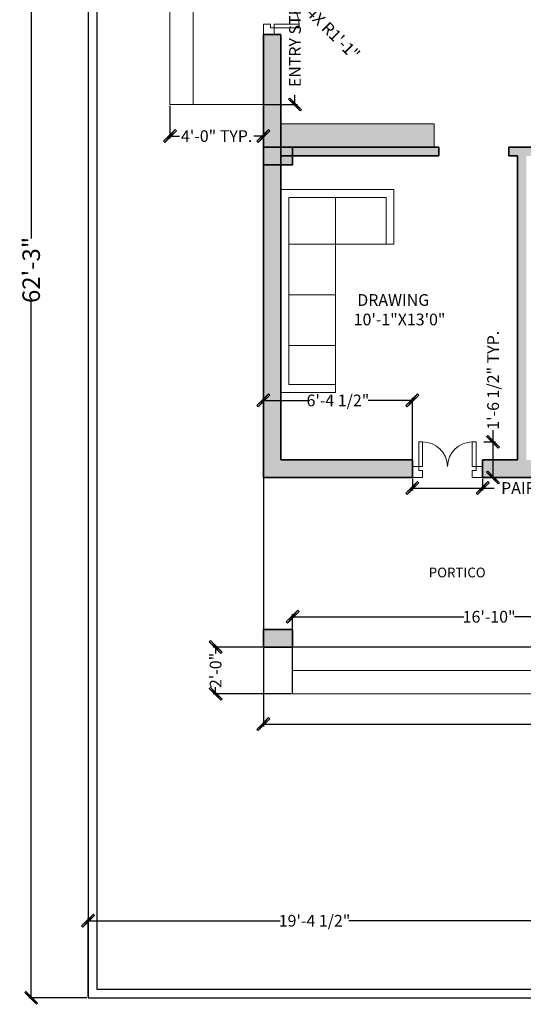
# Model space of a CAD drawing. Units: inches. Extents: x 1018 to 2596, y 723 to 1501.
# Tile 1 of 6: x 1018 to 1276, y 723 to 1229. Entities that reach past the tile are written whole.
import ezdxf

# ---------------------------------------------------------------- set-up
doc = ezdxf.new("R2010")
doc.units = ezdxf.units.IN
doc.layers.get('Defpoints').update_dxf_attribs({"lineweight": 0})
for name, color, linetype, lineweight in [('A-ANNO-DIMS', 2, 'Continuous', 13), ('A-AREA-IDEN', 7, 'Continuous', 18), ('A-COLS', 7, 'Continuous', 35), ('A-DOOR', 4, 'Continuous', 18), ('A-FLOR', 7, 'Continuous', 25), ('A-FLOR-CASE', 8, 'Continuous', 18), ('A-FLOR-CASE-PATT', 9, 'Continuous', 9), ('A-FLOR-STRS', 7, 'Continuous', 18), ('A-FURN', 8, 'Continuous', 13), ('A-WALL', 7, 'Continuous', 35), ('C-PROP', 7, 'Continuous', 25)]:
    doc.layers.add(name, color=color, linetype=linetype, lineweight=lineweight)
doc.layers.add('A-WALL-PATT', color=9, linetype='Continuous', lineweight=9, true_color=0xc7c8ca)
doc.styles.get("Standard").update_dxf_attribs({"font": 'arial.ttf'})
doc.dimstyles.new('saketh', dxfattribs={"dimtxt": 6, "dimasz": 6, "dimexe": 1.25, "dimexo": 0.625, "dimtad": 0, "dimdec": 1, "dimlunit": 4, "dimtxsty": 'Standard', "dimblk": 'ARCHTICK', "dimcen": 2.5, "dimclrd": 256, "dimclre": 1, "dimadec": 0, "dimazin": 0, "dimtfac": 1, "dimtdec": 1, "dimtmove": 0, "dimatfit": 3, "dimldrblk": 'ARCHTICK', "dimfxl": 1, "dimtolj": 1, "dimarcsym": 0})

# ---------------------------------------------------------------- blocks, each defined once
blk = doc.blocks.new('3 1')
at = {"layer": 'A-DOOR'}
for points in [[(-32.72, 5.56), (-32.72, 18.28), (-30.75, 18.28), (-30.75, 5.56)], [(-3.28, 5.56), (-3.28, 18.28), (-5.25, 18.28), (-5.25, 5.56)], [(-32.72, 5.56), (-36, 5.56), (-36, 0), (-30.75, 0), (-30.75, 3.59), (-32.72, 3.59)], [(-5.25, 3.59), (-5.25, 0), (0, 0), (0, 5.56), (-3.28, 5.56), (-3.28, 3.59)]]:
    blk.add_lwpolyline(points, close=True, dxfattribs=at)
at = {"layer": 'A-DOOR', "ltscale": 0.1}
for centre, start, end in [((-30.75, 5.53), 0.1406, 90), ((-5.25, 5.53), 90, 179.8594)]:
    blk.add_arc(centre, 12.75, start, end, dxfattribs=at)
blk = doc.blocks.new('_ArchTick')
for p, q in [((0.447, 0.553), (-0.553, -0.447)), ((-0.447, -0.553), (0.553, 0.447)), ((0.553, 0.447), (0.447, 0.553)), ((-0.553, -0.447), (-0.447, -0.553))]:
    blk.add_line(p, q)
mesh = blk.add_polyface()
corners = [(-0.447, -0.553), (0.447, 0.553), (-0.553, -0.447), (0.553, 0.447)]
mesh.append_faces([[corners[k] for k in face] for face in [(0, 1, 2), (1, 0, 3)]], dxfattribs={"vtx0": -1})
blk = doc.blocks.new('*D49')
at = {"layer": 'A-ANNO-DIMS', "color": 0, "lineweight": -2, "transparency": 16777216}
for p, q in [((1052.06, 1473.73), (1022.21, 1473.73)), ((1023.46, 1473.73), (1023.46, 1116.33)), ((1023.46, 726.73), (1023.46, 1084.12)), ((1052.06, 726.73), (1022.21, 726.73))]:
    blk.add_line(p, q, dxfattribs=at)
at = {"layer": 'Defpoints', "color": 0, "transparency": 16777216}
for p in [(1052.69, 1473.73), (1023.46, 726.73), (1052.69, 726.73)]:
    blk.add_point(p, dxfattribs=at)
at = {"layer": 'A-ANNO-DIMS', "color": 0, "lineweight": -2, "transparency": 16777216, "xscale": 6, "yscale": 6, "zscale": 6}
for p, rotation in [((1023.46, 1473.73), 90), ((1023.46, 726.73), 270)]:
    blk.add_blockref('_ArchTick', p, dxfattribs=dict(at, rotation=rotation))
at = {"layer": 'A-ANNO-DIMS', "color": 0, "transparency": 16777216, "insert": (1023.46, 1100.23), "char_height": 9, "attachment_point": 5, "rotation": 90}
blk.add_mtext('\\A1;62\'-3"', dxfattribs=at)
blk = doc.blocks.new('COLUMN-15X9-IN')
h = blk.add_hatch(color=256)
h.dxf.hatch_style = 1
h.paths.add_polyline_path([(15, 0), (15, 9), (0, 9), (0, 0)])
blk.add_lwpolyline([(15, 9), (15, 0), (0, 0), (0, 9)], close=True)
blk = doc.blocks.new('ENTRY-STEP-108X48-IN')
for p, q in [((0, 0), (0, 108)), ((0, 108), (12, 108)), ((12, 0), (12, 108)), ((48, 108), (12, 108)), ((0, 0), (12, 0)), ((48, 0), (12, 0))]:
    blk.add_line(p, q)
blk = doc.blocks.new('*D59')
at = {"layer": 'A-ANNO-DIMS', "color": 1, "lineweight": -2, "transparency": 16777216}
for p, q in [((1219.19, 993.1), (1219.19, 987.08)), ((1255.19, 993.1), (1255.19, 987.08))]:
    blk.add_line(p, q, dxfattribs=at)
at = {"layer": 'A-ANNO-DIMS', "lineweight": -2, "transparency": 16777216}
for p, q in [((1219.19, 988.33), (1255.19, 988.33)), ((1255.19, 988.33), (1261.19, 988.33))]:
    blk.add_line(p, q, dxfattribs=at)
at = {"layer": 'Defpoints', "color": 0, "transparency": 16777216}
for p in [(1219.19, 993.73), (1255.19, 993.73), (1255.19, 988.33)]:
    blk.add_point(p, dxfattribs=at)
at = {"layer": 'A-ANNO-DIMS', "lineweight": -2, "transparency": 16777216, "xscale": 6, "yscale": 6, "zscale": 6, "rotation": 180}
blk.add_blockref('_ArchTick', (1219.19, 988.33), dxfattribs=at)
at = {"layer": 'A-ANNO-DIMS', "lineweight": -2, "transparency": 16777216, "xscale": 6, "yscale": 6, "zscale": 6}
blk.add_blockref('_ArchTick', (1255.19, 988.33), dxfattribs=at)
at = {"layer": 'A-ANNO-DIMS', "color": 0, "transparency": 16777216, "insert": (1310.45, 988.33), "char_height": 6, "attachment_point": 5}
blk.add_mtext('\\A1;PAIRED DOOR 3\'-0" TYP.', dxfattribs=at)
blk = doc.blocks.new('*D60')
at = {"layer": 'A-ANNO-DIMS', "lineweight": -2, "transparency": 16777216}
for p, q in [((1260.59, 1012.01), (1260.59, 1018.01)), ((1260.59, 993.73), (1260.59, 1012.01))]:
    blk.add_line(p, q, dxfattribs=at)
at = {"layer": 'A-ANNO-DIMS', "color": 1, "lineweight": -2, "transparency": 16777216}
for p, q in [((1255.81, 1012.01), (1261.84, 1012.01)), ((1255.81, 993.73), (1261.84, 993.73))]:
    blk.add_line(p, q, dxfattribs=at)
at = {"layer": 'Defpoints', "color": 0, "transparency": 16777216}
for p in [(1255.19, 1012.01), (1260.59, 1012.01), (1255.19, 993.73)]:
    blk.add_point(p, dxfattribs=at)
at = {"layer": 'A-ANNO-DIMS', "lineweight": -2, "transparency": 16777216, "xscale": 6, "yscale": 6, "zscale": 6}
for p, rotation in [((1260.59, 1012.01), 90), ((1260.59, 993.73), 270)]:
    blk.add_blockref('_ArchTick', p, dxfattribs=dict(at, rotation=rotation))
at = {"layer": 'A-ANNO-DIMS', "color": 0, "transparency": 16777216, "insert": (1260.59, 1043.63), "char_height": 6, "attachment_point": 5, "rotation": 90}
blk.add_mtext('\\A1;1\'-6 1/2" TYP.', dxfattribs=at)
blk = doc.blocks.new('*D69')
at = {"layer": 'A-ANNO-DIMS', "color": 1, "lineweight": -2, "transparency": 16777216}
for p, q in [((1143.31, 1293.11), (1160.14, 1293.11)), ((1143.31, 1185.11), (1160.14, 1185.11))]:
    blk.add_line(p, q, dxfattribs=at)
at = {"layer": 'A-ANNO-DIMS', "lineweight": -2, "transparency": 16777216}
for p, q in [((1158.89, 1293.11), (1158.89, 1288.14)), ((1158.89, 1185.11), (1158.89, 1190.09))]:
    blk.add_line(p, q, dxfattribs=at)
at = {"layer": 'Defpoints', "color": 0, "transparency": 16777216}
for p in [(1142.69, 1293.11), (1158.89, 1293.11), (1142.69, 1185.11)]:
    blk.add_point(p, dxfattribs=at)
at = {"layer": 'A-ANNO-DIMS', "lineweight": -2, "transparency": 16777216, "xscale": 6, "yscale": 6, "zscale": 6}
for p, rotation in [((1158.89, 1293.11), 90), ((1158.89, 1185.11), 270)]:
    blk.add_blockref('_ArchTick', p, dxfattribs=dict(at, rotation=rotation))
at = {"layer": 'A-ANNO-DIMS', "color": 0, "transparency": 16777216, "insert": (1158.89, 1239.11), "char_height": 6, "attachment_point": 5, "rotation": 90}
blk.add_mtext('\\A1;ENTRY STEPS 9\'-0" TYP.', dxfattribs=at)
blk = doc.blocks.new('*D70')
at = {"layer": 'A-ANNO-DIMS', "color": 1, "lineweight": -2, "transparency": 16777216}
for p, q in [((1094.69, 1184.49), (1094.69, 1167.66)), ((1142.69, 1184.49), (1142.69, 1167.66))]:
    blk.add_line(p, q, dxfattribs=at)
at = {"layer": 'A-ANNO-DIMS', "lineweight": -2, "transparency": 16777216}
for p, q in [((1094.69, 1168.91), (1099.65, 1168.91)), ((1142.69, 1168.91), (1137.72, 1168.91))]:
    blk.add_line(p, q, dxfattribs=at)
at = {"layer": 'Defpoints', "color": 0, "transparency": 16777216}
for p in [(1094.69, 1185.11), (1142.69, 1185.11), (1142.69, 1168.91)]:
    blk.add_point(p, dxfattribs=at)
at = {"layer": 'A-ANNO-DIMS', "lineweight": -2, "transparency": 16777216, "xscale": 6, "yscale": 6, "zscale": 6, "rotation": 180}
blk.add_blockref('_ArchTick', (1094.69, 1168.91), dxfattribs=at)
at = {"layer": 'A-ANNO-DIMS', "lineweight": -2, "transparency": 16777216, "xscale": 6, "yscale": 6, "zscale": 6}
blk.add_blockref('_ArchTick', (1142.69, 1168.91), dxfattribs=at)
at = {"layer": 'A-ANNO-DIMS', "color": 0, "transparency": 16777216, "insert": (1118.69, 1168.91), "char_height": 6, "attachment_point": 5}
blk.add_mtext('\\A1;4\'-0" TYP.', dxfattribs=at)
blk = doc.blocks.new('*D79')
at = {"layer": 'A-ANNO-DIMS', "color": 1, "lineweight": -2, "transparency": 16777216}
for p, q in [((1142.69, 906.1), (1142.69, 865.93)), ((1583.69, 906.1), (1583.69, 865.93))]:
    blk.add_line(p, q, dxfattribs=at)
at = {"layer": 'A-ANNO-DIMS', "lineweight": -2, "transparency": 16777216}
for p, q in [((1142.69, 867.18), (1352.26, 867.18)), ((1583.69, 867.18), (1374.12, 867.18))]:
    blk.add_line(p, q, dxfattribs=at)
at = {"layer": 'Defpoints', "color": 0, "transparency": 16777216}
for p in [(1142.69, 906.73), (1583.69, 906.73), (1142.69, 867.18)]:
    blk.add_point(p, dxfattribs=at)
at = {"layer": 'A-ANNO-DIMS', "lineweight": -2, "transparency": 16777216, "xscale": 6, "yscale": 6, "zscale": 6, "rotation": 180}
blk.add_blockref('_ArchTick', (1142.69, 867.18), dxfattribs=at)
at = {"layer": 'A-ANNO-DIMS', "lineweight": -2, "transparency": 16777216, "xscale": 6, "yscale": 6, "zscale": 6}
blk.add_blockref('_ArchTick', (1583.69, 867.18), dxfattribs=at)
at = {"layer": 'A-ANNO-DIMS', "color": 0, "transparency": 16777216, "insert": (1363.19, 867.18), "char_height": 6, "attachment_point": 5}
blk.add_mtext('\\A1;36\'-9"', dxfattribs=at)
blk = doc.blocks.new('*D82')
at = {"layer": 'A-ANNO-DIMS', "color": 1, "lineweight": -2, "transparency": 16777216}
for p, q in [((1052.69, 727.35), (1052.69, 767.53)), ((1285.19, 727.35), (1285.19, 767.53))]:
    blk.add_line(p, q, dxfattribs=at)
at = {"layer": 'A-ANNO-DIMS', "lineweight": -2, "transparency": 16777216}
for p, q in [((1052.69, 766.28), (1151.3, 766.28)), ((1285.19, 766.28), (1186.58, 766.28))]:
    blk.add_line(p, q, dxfattribs=at)
at = {"layer": 'Defpoints', "color": 0, "transparency": 16777216}
for p in [(1285.19, 766.28), (1052.69, 726.73), (1285.19, 726.73)]:
    blk.add_point(p, dxfattribs=at)
at = {"layer": 'A-ANNO-DIMS', "lineweight": -2, "transparency": 16777216, "xscale": 6, "yscale": 6, "zscale": 6, "rotation": 180}
blk.add_blockref('_ArchTick', (1052.69, 766.28), dxfattribs=at)
at = {"layer": 'A-ANNO-DIMS', "lineweight": -2, "transparency": 16777216, "xscale": 6, "yscale": 6, "zscale": 6}
blk.add_blockref('_ArchTick', (1285.19, 766.28), dxfattribs=at)
at = {"layer": 'A-ANNO-DIMS', "color": 0, "transparency": 16777216, "insert": (1168.94, 766.28), "char_height": 6, "attachment_point": 5}
blk.add_mtext('\\A1;19\'-4 1/2"', dxfattribs=at)
blk = doc.blocks.new('*D84')
at = {"layer": 'A-ANNO-DIMS', "color": 1, "lineweight": -2, "transparency": 16777216}
for p, q in [((1157.69, 883.35), (1157.69, 923.53)), ((1359.46, 883.35), (1359.46, 923.53))]:
    blk.add_line(p, q, dxfattribs=at)
at = {"layer": 'A-ANNO-DIMS', "lineweight": -2, "transparency": 16777216}
for p, q in [((1157.69, 922.28), (1245.6, 922.28)), ((1359.46, 922.28), (1271.55, 922.28))]:
    blk.add_line(p, q, dxfattribs=at)
at = {"layer": 'Defpoints', "color": 0, "transparency": 16777216}
for p in [(1359.46, 922.28), (1157.69, 882.73), (1359.46, 882.73)]:
    blk.add_point(p, dxfattribs=at)
at = {"layer": 'A-ANNO-DIMS', "lineweight": -2, "transparency": 16777216, "xscale": 6, "yscale": 6, "zscale": 6, "rotation": 180}
blk.add_blockref('_ArchTick', (1157.69, 922.28), dxfattribs=at)
at = {"layer": 'A-ANNO-DIMS', "lineweight": -2, "transparency": 16777216, "xscale": 6, "yscale": 6, "zscale": 6}
blk.add_blockref('_ArchTick', (1359.46, 922.28), dxfattribs=at)
at = {"layer": 'A-ANNO-DIMS', "color": 0, "transparency": 16777216, "insert": (1258.57, 922.28), "char_height": 6, "attachment_point": 5}
blk.add_mtext('\\A1;16\'-10"', dxfattribs=at)
blk = doc.blocks.new('*D85')
at = {"layer": 'A-ANNO-DIMS', "color": 1, "lineweight": -2, "transparency": 16777216}
for p, q in [((1157.06, 906.73), (1116.89, 906.73)), ((1157.06, 882.73), (1116.89, 882.73))]:
    blk.add_line(p, q, dxfattribs=at)
at = {"layer": 'A-ANNO-DIMS', "lineweight": -2, "transparency": 16777216}
for p, q in [((1118.14, 906.73), (1118.14, 903.38)), ((1118.14, 882.73), (1118.14, 886.07))]:
    blk.add_line(p, q, dxfattribs=at)
at = {"layer": 'Defpoints', "color": 0, "transparency": 16777216}
for p in [(1118.14, 906.73), (1157.69, 906.73), (1157.69, 882.73)]:
    blk.add_point(p, dxfattribs=at)
at = {"layer": 'A-ANNO-DIMS', "lineweight": -2, "transparency": 16777216, "xscale": 6, "yscale": 6, "zscale": 6}
for p, rotation in [((1118.14, 906.73), 90), ((1118.14, 882.73), 270)]:
    blk.add_blockref('_ArchTick', p, dxfattribs=dict(at, rotation=rotation))
at = {"layer": 'A-ANNO-DIMS', "color": 0, "transparency": 16777216, "insert": (1118.14, 894.73), "char_height": 6, "attachment_point": 5, "rotation": 90}
blk.add_mtext('\\A1;2\'-0"', dxfattribs=at)
blk = doc.blocks.new('*D88')
at = {"layer": 'A-ANNO-DIMS', "color": 1, "lineweight": -2, "transparency": 16777216}
for p, q in [((1142.69, 994.35), (1142.69, 1034.53)), ((1219.19, 994.35), (1219.19, 1034.53))]:
    blk.add_line(p, q, dxfattribs=at)
at = {"layer": 'A-ANNO-DIMS', "lineweight": -2, "transparency": 16777216}
for p, q in [((1142.69, 1033.28), (1165.33, 1033.28)), ((1219.19, 1033.28), (1196.54, 1033.28))]:
    blk.add_line(p, q, dxfattribs=at)
at = {"layer": 'Defpoints', "color": 0, "transparency": 16777216}
for p in [(1219.19, 1033.28), (1142.69, 993.73), (1219.19, 993.73)]:
    blk.add_point(p, dxfattribs=at)
at = {"layer": 'A-ANNO-DIMS', "lineweight": -2, "transparency": 16777216, "xscale": 6, "yscale": 6, "zscale": 6, "rotation": 180}
blk.add_blockref('_ArchTick', (1142.69, 1033.28), dxfattribs=at)
at = {"layer": 'A-ANNO-DIMS', "lineweight": -2, "transparency": 16777216, "xscale": 6, "yscale": 6, "zscale": 6}
blk.add_blockref('_ArchTick', (1219.19, 1033.28), dxfattribs=at)
at = {"layer": 'A-ANNO-DIMS', "color": 0, "transparency": 16777216, "insert": (1180.94, 1033.28), "char_height": 6, "attachment_point": 5}
blk.add_mtext('\\A1;6\'-4 1/2"', dxfattribs=at)
blk = doc.blocks.new('*D117')
at = {"layer": 'A-ANNO-DIMS', "lineweight": -2, "transparency": 16777216}
for p in [(1148.22, 1251.86), (1165.74, 1234.39)]:
    blk.add_line(p, (1157.25, 1242.86), dxfattribs=at)
at = {"layer": 'Defpoints', "color": 0, "transparency": 16777216}
for p in [(1148.22, 1251.86), (1157.25, 1242.86)]:
    blk.add_point(p, dxfattribs=at)
at = {"layer": 'A-ANNO-DIMS', "lineweight": -2, "transparency": 16777216, "xscale": 6, "yscale": 6, "zscale": 6, "rotation": 135.0720928995186}
blk.add_blockref('_ArchTick', (1157.25, 1242.86), dxfattribs=at)
at = {"layer": 'A-ANNO-DIMS', "color": 0, "transparency": 16777216, "insert": (1178.51, 1221.65), "char_height": 6, "attachment_point": 5, "rotation": 315.0721}
blk.add_mtext('\\A1;4X R1\'-1"', dxfattribs=at)

msp = doc.modelspace()

# ---------------------------------------------------------------- hatches: boundary and pattern name
at = {"layer": 'A-FLOR-CASE-PATT', "transparency": 33554531}
h = msp.add_hatch(color=256, dxfattribs=at)
h.dxf.hatch_style = 1
h.paths.add_polyline_path([(1230.28, 1175.23), (1151.69, 1175.23), (1151.69, 1163.23), (1230.28, 1163.23)])
at = {"layer": 'A-WALL-PATT', "transparency": 33554539}
h = msp.add_hatch(color=256, dxfattribs=at)
h.dxf.hatch_style = 1
h.paths.add_polyline_path([(1359.46, 1344.73), (1359.46, 1353.73), (1322.14, 1353.73), (1322.14, 1348.16), (1322.14, 1344.73)])
h.paths.add_polyline_path([(1374.46, 1353.73), (1374.46, 1344.73), (1421.69, 1344.73), (1421.69, 1296.73), (1415.69, 1296.73), (1415.69, 1292.23), (1426.19, 1292.23), (1426.19, 1344.73), (1568.69, 1344.73), (1568.69, 1353.73)])
h.paths.add_polyline_path([(1257.69, 1344.73), (1274.14, 1344.73), (1274.14, 1353.73), (1157.69, 1353.73), (1157.69, 1344.73)])
h.paths.add_polyline_path([(1151.69, 1344.73), (1142.69, 1344.73), (1142.69, 1257.11), (1148.25, 1257.11), (1151.69, 1257.11)])
h.paths.add_polyline_path([(1142.69, 1163.23), (1151.69, 1163.23), (1151.69, 1221.11), (1142.69, 1221.11)])
h.paths.add_polyline_path([(1151.69, 1154.23), (1142.69, 1154.23), (1142.69, 993.73), (1219.19, 993.73), (1219.19, 999.29), (1219.19, 1002.73), (1151.69, 1002.73)])
h.paths.add_polyline_path([(1327.94, 993.73), (1327.94, 1002.73), (1277.69, 1002.73), (1277.69, 1158.73), (1283.22, 1158.73), (1283.22, 1163.23), (1273.19, 1163.23), (1268.69, 1163.23), (1268.69, 1158.73), (1273.19, 1158.73), (1273.19, 1002.73), (1255.19, 1002.73), (1255.19, 993.73)])
h.paths.add_polyline_path([(1426.19, 1002.73), (1426.19, 1178.23), (1421.69, 1178.23), (1421.69, 1163.23), (1374.46, 1163.23), (1374.46, 1158.73), (1421.69, 1158.73), (1421.69, 1002.73), (1375.94, 1002.73), (1375.94, 993.73), (1478.69, 993.73), (1478.69, 1002.73)])
h.paths.add_polyline_path([(1583.69, 1233.73), (1574.69, 1233.73), (1574.69, 1229.23), (1421.69, 1229.23), (1421.69, 1220.23), (1426.19, 1220.23), (1426.19, 1224.73), (1480.19, 1224.73), (1480.19, 1158.73), (1489.19, 1158.73), (1489.19, 1163.23), (1484.69, 1163.23), (1484.69, 1224.73), (1508.69, 1224.73), (1574.69, 1224.73), (1574.69, 1163.23), (1583.69, 1163.23)])
h.paths.add_polyline_path([(1574.69, 1263.73), (1580.52, 1263.73), (1583.69, 1263.73), (1583.69, 1344.73), (1574.69, 1344.73)])
h.paths.add_polyline_path([(1583.69, 1154.23), (1574.69, 1154.23), (1574.69, 1002.73), (1583.69, 1002.73)])
h.paths.add_polyline_path([(1568.69, 993.73), (1568.69, 1002.73), (1526.69, 1002.73), (1526.69, 993.73)])
h.paths.add_polyline_path([(1359.46, 1158.73), (1359.46, 1163.23), (1325.22, 1163.23), (1325.22, 1158.73)])
h.paths.add_polyline_path([(1232.69, 1158.73), (1232.69, 1163.23), (1157.69, 1163.23), (1157.69, 1158.73)])

# ---------------------------------------------------------------- linework, layer by layer
at = {"layer": 'A-FLOR'}
for p in [(1142.69, 993.73), (1374.46, 906.73)]:
    msp.add_line(p, (1142.69, 906.73), dxfattribs=at)
at = {"layer": 'A-FLOR-CASE'}
for q in [(1151.69, 1175.23), (1230.28, 1163.23)]:
    msp.add_line((1230.28, 1175.23), q, dxfattribs=at)
at = {"layer": 'A-FLOR-STRS'}
for p, q in [((1157.69, 906.73), (1157.69, 882.73)), ((1359.46, 894.73), (1157.69, 894.73)), ((1359.46, 882.73), (1157.69, 882.73))]:
    msp.add_line(p, q, dxfattribs=at)
at = {"layer": 'A-FURN'}
for p, q in [((1151.69, 1037.42), (1151.69, 1141.42)), ((1151.69, 1141.42), (1209.69, 1141.42)), ((1155.69, 1041.42), (1155.69, 1137.42)), ((1155.69, 1137.42), (1205.69, 1137.42)), ((1179.69, 1037.42), (1179.69, 1137.42)), ((1205.69, 1113.42), (1205.69, 1137.42)), ((1209.69, 1141.42), (1209.69, 1137.42)), ((1209.69, 1113.42), (1209.69, 1137.42)), ((1155.69, 1113.42), (1209.69, 1113.42)), ((1155.69, 1087.42), (1179.69, 1087.42)), ((1155.69, 1061.42), (1179.69, 1061.42)), ((1179.69, 1041.42), (1155.69, 1041.42)), ((1179.69, 1037.42), (1151.69, 1037.42))]:
    msp.add_line(p, q, dxfattribs=at)
at = {"layer": 'A-WALL'}
for p, q in [((1142.69, 993.73), (1142.69, 1221.11)), ((1151.69, 1221.11), (1142.69, 1221.11)), ((1151.69, 1002.73), (1151.69, 1221.11)), ((1232.69, 1163.23), (1151.69, 1163.23)), ((1232.69, 1158.73), (1232.69, 1163.23)), ((1273.19, 1163.23), (1268.69, 1163.23)), ((1268.69, 1158.73), (1268.69, 1163.23)), ((1273.19, 1163.23), (1283.22, 1163.23)), ((1232.69, 1158.73), (1151.69, 1158.73)), ((1273.19, 1158.73), (1268.69, 1158.73)), ((1273.19, 1158.73), (1273.19, 1002.73)), ((1219.19, 1002.73), (1151.69, 1002.73)), ((1219.19, 1002.73), (1219.19, 993.73)), ((1273.19, 1002.73), (1255.19, 1002.73)), ((1255.19, 1002.73), (1255.19, 993.73)), ((1219.19, 993.73), (1142.69, 993.73)), ((1327.94, 993.73), (1255.19, 993.73))]:
    msp.add_line(p, q, dxfattribs=at)
at = {"layer": 'C-PROP'}
for points in [[(1405.19, 726.73), (1637.69, 726.73), (1637.69, 1473.73), (1052.69, 1473.73), (1052.69, 726.73), (1285.19, 726.73)], [(1405.19, 731.23), (1633.19, 731.23), (1633.19, 1469.23), (1057.19, 1469.23), (1057.19, 731.23), (1285.19, 731.23)]]:
    msp.add_lwpolyline(points, dxfattribs=at)

# ---------------------------------------------------------------- block references
at = {"layer": 'A-COLS'}
for p in [(1142.69, 1154.22), (1142.69, 906.72)]:
    msp.add_blockref('COLUMN-15X9-IN', p, dxfattribs=at)
at = {"layer": 'A-DOOR', "rotation": 270}
msp.add_blockref('3 1', (1142.69, 1221.11), dxfattribs=at)
at = {"layer": 'A-DOOR'}
msp.add_blockref('3 1', (1255.19, 993.73), dxfattribs=at)
at = {"layer": 'A-FLOR-STRS'}
msp.add_blockref('ENTRY-STEP-108X48-IN', (1094.69, 1185.11), dxfattribs=at)

# ---------------------------------------------------------------- texts
at = {"layer": 'A-AREA-IDEN', "attachment_point": 1}
for s, width, insert, char_height in [('\\A1;{\\H0.66667x;    DRAWING\\P   10\'-1"X13\'0"}', 129.8331, (1183.53, 1087.8), 9), ('\\A1;PORTICO', 100.7198, (1227.57, 947.48), 5)]:
    msp.add_mtext_dynamic_manual_height_columns(s, width=width, gutter_width=12.5, heights=[0], dxfattribs=dict(at, insert=insert, char_height=char_height))

# ---------------------------------------------------------------- dimensions: what is measured, and where the dimension line sits
at = {"layer": 'A-ANNO-DIMS'}
dim = msp.add_linear_dim(base=(1023.46, 726.73), p1=(1052.69, 1473.73), p2=(1052.69, 726.73), angle=90, dimstyle='saketh', override={"dimtxt": 9, "dimclrd": 0, "dimclre": 0, "dimclrt": 0}, dxfattribs=at)
dim.commit()
dim.dimension.update_dxf_attribs({"geometry": '*D49', "text_midpoint": (1023.46, 1100.23), "dimtype": 160})
for base, p1, p2, text, picture, middle in [((1158.89, 1293.11), (1142.69, 1185.11), (1142.69, 1293.11), 'ENTRY STEPS <> TYP.', '*D69', (1158.89, 1239.11)), ((1260.59, 1012.01), (1255.19, 993.73), (1255.19, 1012.01), '<> TYP.', '*D60', (1260.59, 1043.63))]:
    dim = msp.add_linear_dim(base=base, p1=p1, p2=p2, angle=90, text=text, dimstyle='saketh', override={"dimdec": 1, "dimlfac": 1, "dimrnd": 0, "dimzin": 1, "dimdsep": 46, "dimlunit": 4, "dimfrac": 2}, dxfattribs=at)
    dim.commit()
    dim.dimension.update_dxf_attribs({"geometry": picture, "text_midpoint": middle})
dim = msp.add_radius_dim(center=(1148.21807, 1251.86424), mpoint=(1157.24504, 1242.85996), text='4X <>', dimstyle='saketh', override={"dimdec": 1, "dimlfac": 1, "dimrnd": 0, "dimzin": 1, "dimdsep": 46, "dimlunit": 4, "dimfrac": 2}, dxfattribs=at)
dim.commit()
dim.dimension.update_dxf_attribs({"geometry": '*D117', "text_midpoint": (1178.5116, 1221.64685)})
for base, p1, p2, text, picture, middle in [((1142.69, 1168.91), (1094.69, 1185.11), (1142.69, 1185.11), '<> TYP.', '*D70', (1118.69, 1168.91)), ((1255.19, 988.33), (1219.19, 993.73), (1255.19, 993.73), 'PAIRED DOOR <> TYP.', '*D59', (1310.45, 988.33))]:
    dim = msp.add_linear_dim(base=base, p1=p1, p2=p2, text=text, dimstyle='saketh', override={"dimdec": 1, "dimlfac": 1, "dimrnd": 0, "dimzin": 1, "dimdsep": 46, "dimlunit": 4, "dimfrac": 2}, dxfattribs=at)
    dim.commit()
    dim.dimension.update_dxf_attribs({"geometry": picture, "text_midpoint": middle})
for base, p1, p2, picture, middle in [((1219.19, 1033.28), (1142.69, 993.73), (1219.19, 993.73), '*D88', (1180.94, 1033.28)), ((1359.46, 922.28), (1157.69, 882.73), (1359.46, 882.73), '*D84', (1258.57, 922.28)), ((1285.19, 766.28), (1052.69, 726.73), (1285.19, 726.73), '*D82', (1168.94, 766.28))]:
    dim = msp.add_linear_dim(base=base, p1=p1, p2=p2, dimstyle='saketh', override={"dimdec": 1, "dimlfac": 1, "dimrnd": 0, "dimzin": 1, "dimdsep": 46, "dimlunit": 4, "dimfrac": 2}, dxfattribs=at)
    dim.commit()
    dim.dimension.update_dxf_attribs({"geometry": picture, "text_midpoint": middle})
for base, p1, p2, angle, picture, middle in [((1118.14, 906.73), (1157.69, 882.73), (1157.69, 906.73), 90, '*D85', (1118.14, 894.73)), ((1142.69, 867.18), (1583.69, 906.73), (1142.69, 906.73), 180, '*D79', (1363.19, 867.18))]:
    dim = msp.add_linear_dim(base=base, p1=p1, p2=p2, angle=angle, dimstyle='saketh', override={"dimdec": 1, "dimlfac": 1, "dimrnd": 0, "dimzin": 1, "dimdsep": 46, "dimlunit": 4, "dimfrac": 2}, dxfattribs=at)
    dim.commit()
    dim.dimension.update_dxf_attribs({"geometry": picture, "text_midpoint": middle})

doc.saveas('drawing.dxf')
